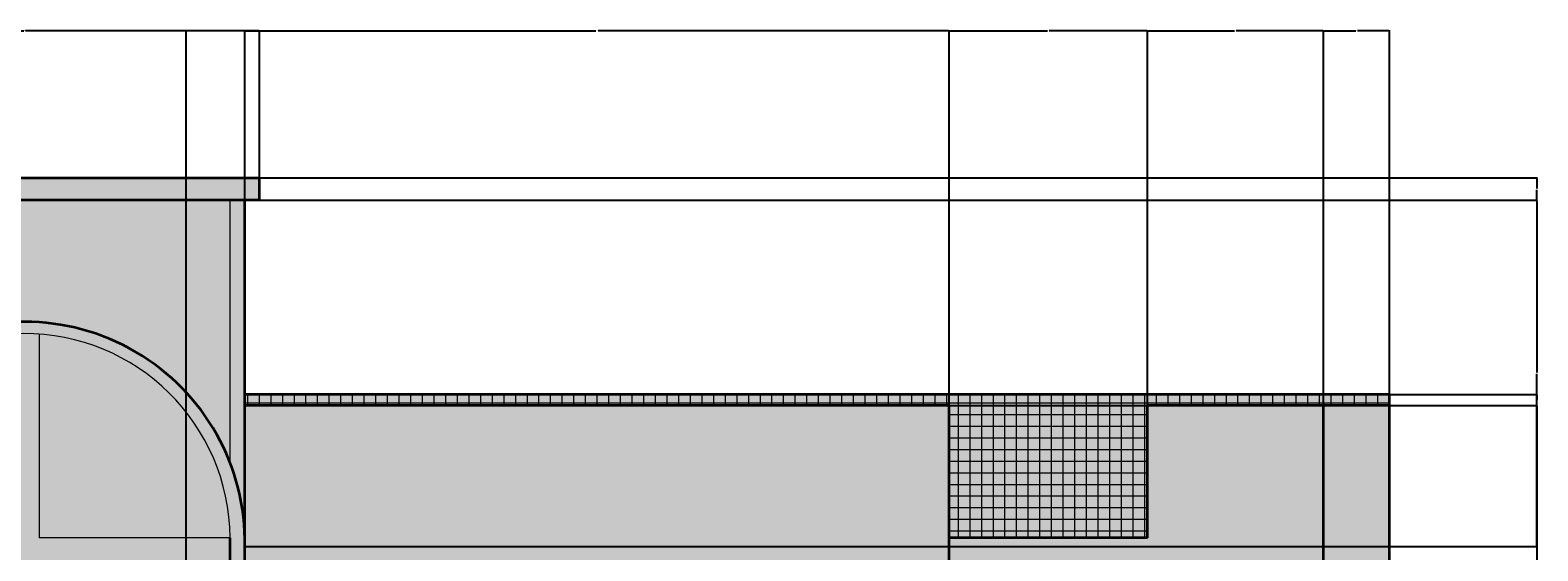
# Model space of a CAD drawing. Units: inches. Extents: x 2794 to 3619, y 522 to 1397.
# Tile 10 of 10: x 3208 to 3619, y 1255 to 1397. Entities that reach past the tile are written whole.
import ezdxf

# ---------------------------------------------------------------- set-up
doc = ezdxf.new("R2010")
doc.units = ezdxf.units.IN
for name, color, linetype, lineweight in [('A-ANNO-DIMS', 2, 'Continuous', 18), ('A-ELEV', 7, 'Continuous', 35), ('A-ELEV-PATT', 8, 'Continuous', 13), ('A-GLAZ', 4, 'Continuous', 18)]:
    doc.layers.add(name, color=color, linetype=linetype, lineweight=lineweight)
doc.styles.get("Standard").update_dxf_attribs({"font": 'arial.ttf'})
doc.dimstyles.get("Standard").update_dxf_attribs({"dimtxt": 0.18, "dimasz": 0.18, "dimexe": 0.18, "dimexo": 0.0625, "dimgap": 0.09, "dimtad": 0, "dimtih": 1, "dimtoh": 1, "dimdec": 4, "dimzin": 0, "dimdsep": 46, "dimtxsty": 'Standard', "dimcen": 0.09, "dimadec": 0, "dimazin": 0, "dimtfac": 1, "dimtdec": 4, "dimtofl": 0, "dimtmove": 0, "dimatfit": 3, "dimfxl": 1, "dimtolj": 1, "dimtzin": 0, "dimarcsym": 0})

# ---------------------------------------------------------------- blocks, each defined once
blk = doc.blocks.new('*D12')
at = {"layer": 'A-ANNO-DIMS', "color": 0, "lineweight": -2, "transparency": 16777216}
for p, q in [((3266.27, 1294.7), (3266.27, 1396.92)), ((3266.45, 1396.74), (3361.99, 1396.74)), ((3458.09, 1396.74), (3362.55, 1396.74)), ((3458.27, 1294.7), (3458.27, 1396.92))]:
    blk.add_line(p, q, dxfattribs=at)
at = {"layer": 'A-ANNO-DIMS', "color": 0, "transparency": 16777216}
for points in [[(3266.45, 1396.77), (3266.45, 1396.71), (3266.27, 1396.74)], [(3458.09, 1396.77), (3458.09, 1396.71), (3458.27, 1396.74)]]:
    blk.add_solid(points, dxfattribs=at)
at = {"layer": 'Defpoints', "color": 0, "transparency": 16777216}
for p in [(3458.27, 1396.74), (3266.27, 1294.64), (3458.27, 1294.64)]:
    blk.add_point(p, dxfattribs=at)
at = {"layer": 'A-ANNO-DIMS', "color": 0, "transparency": 16777216, "insert": (3362.27, 1396.74), "char_height": 0.18, "attachment_point": 5}
blk.add_mtext('\\A1;192', dxfattribs=at)
blk = doc.blocks.new('*D13')
at = {"layer": 'A-ANNO-DIMS', "color": 0, "lineweight": -2, "transparency": 16777216}
for p, q in [((3458.27, 1294.7), (3458.27, 1396.92)), ((3458.45, 1396.74), (3485.05, 1396.74)), ((3512.09, 1396.74), (3485.48, 1396.74)), ((3512.27, 1294.7), (3512.27, 1396.92))]:
    blk.add_line(p, q, dxfattribs=at)
at = {"layer": 'A-ANNO-DIMS', "color": 0, "transparency": 16777216}
for points in [[(3458.45, 1396.77), (3458.45, 1396.71), (3458.27, 1396.74)], [(3512.09, 1396.77), (3512.09, 1396.71), (3512.27, 1396.74)]]:
    blk.add_solid(points, dxfattribs=at)
at = {"layer": 'Defpoints', "color": 0, "transparency": 16777216}
for p in [(3512.27, 1396.74), (3458.27, 1294.64), (3512.27, 1294.64)]:
    blk.add_point(p, dxfattribs=at)
at = {"layer": 'A-ANNO-DIMS', "color": 0, "transparency": 16777216, "insert": (3485.27, 1396.74), "char_height": 0.18, "attachment_point": 5}
blk.add_mtext('\\A1;54', dxfattribs=at)
blk = doc.blocks.new('*D14')
at = {"layer": 'A-ANNO-DIMS', "color": 0, "lineweight": -2, "transparency": 16777216}
for p, q in [((3512.27, 1294.7), (3512.27, 1396.92)), ((3512.45, 1396.74), (3536.04, 1396.74)), ((3560.09, 1396.74), (3536.49, 1396.74)), ((3560.27, 1294.7), (3560.27, 1396.92))]:
    blk.add_line(p, q, dxfattribs=at)
at = {"layer": 'A-ANNO-DIMS', "color": 0, "transparency": 16777216}
for points in [[(3512.45, 1396.77), (3512.45, 1396.71), (3512.27, 1396.74)], [(3560.09, 1396.77), (3560.09, 1396.71), (3560.27, 1396.74)]]:
    blk.add_solid(points, dxfattribs=at)
at = {"layer": 'Defpoints', "color": 0, "transparency": 16777216}
for p in [(3560.27, 1396.74), (3512.27, 1294.64), (3560.27, 1294.64)]:
    blk.add_point(p, dxfattribs=at)
at = {"layer": 'A-ANNO-DIMS', "color": 0, "transparency": 16777216, "insert": (3536.27, 1396.74), "char_height": 0.18, "attachment_point": 5}
blk.add_mtext('\\A1;48', dxfattribs=at)
blk = doc.blocks.new('*D15')
at = {"layer": 'A-ANNO-DIMS', "color": 0, "lineweight": -2, "transparency": 16777216}
for p, q in [((3560.27, 1294.7), (3560.27, 1396.92)), ((3560.45, 1396.74), (3569.06, 1396.74)), ((3578.09, 1396.74), (3569.48, 1396.74)), ((3578.27, 1294.7), (3578.27, 1396.92))]:
    blk.add_line(p, q, dxfattribs=at)
at = {"layer": 'A-ANNO-DIMS', "color": 0, "transparency": 16777216}
for points in [[(3560.45, 1396.77), (3560.45, 1396.71), (3560.27, 1396.74)], [(3578.09, 1396.77), (3578.09, 1396.71), (3578.27, 1396.74)]]:
    blk.add_solid(points, dxfattribs=at)
at = {"layer": 'Defpoints', "color": 0, "transparency": 16777216}
for p in [(3578.27, 1396.74), (3560.27, 1294.64), (3578.27, 1294.64)]:
    blk.add_point(p, dxfattribs=at)
at = {"layer": 'A-ANNO-DIMS', "color": 0, "transparency": 16777216, "insert": (3569.27, 1396.74), "char_height": 0.18, "attachment_point": 5}
blk.add_mtext('\\A1;18', dxfattribs=at)
blk = doc.blocks.new('*D23')
at = {"layer": 'A-ANNO-DIMS', "color": 0, "lineweight": -2, "transparency": 16777216}
for p, q in [((3458.33, 1294.64), (3618.55, 1294.64)), ((3618.37, 1294.46), (3618.37, 1232.82)), ((3618.37, 1170.82), (3618.37, 1232.45)), ((3458.33, 1170.64), (3618.55, 1170.64))]:
    blk.add_line(p, q, dxfattribs=at)
at = {"layer": 'A-ANNO-DIMS', "color": 0, "transparency": 16777216}
for points in [[(3618.34, 1294.46), (3618.4, 1294.46), (3618.37, 1294.64)], [(3618.34, 1170.82), (3618.4, 1170.82), (3618.37, 1170.64)]]:
    blk.add_solid(points, dxfattribs=at)
at = {"layer": 'Defpoints', "color": 0, "transparency": 16777216}
for p in [(3458.27, 1294.64), (3618.37, 1294.64), (3458.27, 1170.64)]:
    blk.add_point(p, dxfattribs=at)
at = {"layer": 'A-ANNO-DIMS', "color": 0, "transparency": 16777216, "insert": (3618.37, 1232.64), "char_height": 0.18, "attachment_point": 5}
blk.add_mtext('\\A1;124', dxfattribs=at)
blk = doc.blocks.new('*D24')
at = {"layer": 'A-ANNO-DIMS', "color": 0, "lineweight": -2, "transparency": 16777216}
for p, q in [((3578.33, 1297.64), (3618.55, 1297.64)), ((3578.33, 1294.64), (3618.55, 1294.64)), ((3618.37, 1297.46), (3618.37, 1296.32)), ((3618.37, 1294.82), (3618.37, 1295.95))]:
    blk.add_line(p, q, dxfattribs=at)
at = {"layer": 'A-ANNO-DIMS', "color": 0, "transparency": 16777216}
for points in [[(3618.34, 1297.46), (3618.4, 1297.46), (3618.37, 1297.64)], [(3618.34, 1294.82), (3618.4, 1294.82), (3618.37, 1294.64)]]:
    blk.add_solid(points, dxfattribs=at)
at = {"layer": 'Defpoints', "color": 0, "transparency": 16777216}
for p in [(3578.27, 1297.64), (3578.27, 1294.64), (3618.37, 1297.64)]:
    blk.add_point(p, dxfattribs=at)
at = {"layer": 'A-ANNO-DIMS', "color": 0, "transparency": 16777216, "insert": (3618.37, 1296.14), "char_height": 0.18, "attachment_point": 5}
blk.add_mtext('\\A1;3', dxfattribs=at)
blk = doc.blocks.new('*D44')
at = {"layer": 'A-ANNO-DIMS', "color": 0, "lineweight": -2, "transparency": 16777216}
for p, q in [((3142.27, 1356.7), (3142.27, 1396.92)), ((3142.45, 1396.74), (3205.99, 1396.74)), ((3270.09, 1396.74), (3206.55, 1396.74)), ((3270.27, 1356.7), (3270.27, 1396.92))]:
    blk.add_line(p, q, dxfattribs=at)
at = {"layer": 'A-ANNO-DIMS', "color": 0, "transparency": 16777216}
for points in [[(3142.45, 1396.77), (3142.45, 1396.71), (3142.27, 1396.74)], [(3270.09, 1396.77), (3270.09, 1396.71), (3270.27, 1396.74)]]:
    blk.add_solid(points, dxfattribs=at)
at = {"layer": 'Defpoints', "color": 0, "transparency": 16777216}
for p in [(3270.27, 1396.74), (3142.27, 1356.64), (3270.27, 1356.64)]:
    blk.add_point(p, dxfattribs=at)
at = {"layer": 'A-ANNO-DIMS', "color": 0, "transparency": 16777216, "insert": (3206.27, 1396.74), "char_height": 0.18, "attachment_point": 5}
blk.add_mtext('\\A1;128', dxfattribs=at)
blk = doc.blocks.new('*D45')
at = {"layer": 'A-ANNO-DIMS', "color": 0, "lineweight": -2, "transparency": 16777216}
for p, q in [((3146.27, 1350.7), (3146.27, 1396.92)), ((3146.45, 1396.74), (3205.99, 1396.74)), ((3266.09, 1396.74), (3206.55, 1396.74)), ((3266.27, 1350.7), (3266.27, 1396.92))]:
    blk.add_line(p, q, dxfattribs=at)
at = {"layer": 'A-ANNO-DIMS', "color": 0, "transparency": 16777216}
for points in [[(3146.45, 1396.77), (3146.45, 1396.71), (3146.27, 1396.74)], [(3266.09, 1396.77), (3266.09, 1396.71), (3266.27, 1396.74)]]:
    blk.add_solid(points, dxfattribs=at)
at = {"layer": 'Defpoints', "color": 0, "transparency": 16777216}
for p in [(3266.27, 1396.74), (3146.27, 1350.64), (3266.27, 1350.64)]:
    blk.add_point(p, dxfattribs=at)
at = {"layer": 'A-ANNO-DIMS', "color": 0, "transparency": 16777216, "insert": (3206.27, 1396.74), "char_height": 0.18, "attachment_point": 5}
blk.add_mtext('\\A1;120', dxfattribs=at)
blk = doc.blocks.new('*D46')
at = {"layer": 'A-ANNO-DIMS', "color": 0, "lineweight": -2, "transparency": 16777216}
for p, q in [((3270.33, 1356.64), (3618.55, 1356.64)), ((3618.37, 1356.46), (3618.37, 1353.82)), ((3618.37, 1350.82), (3618.37, 1353.45)), ((3270.33, 1350.64), (3618.55, 1350.64))]:
    blk.add_line(p, q, dxfattribs=at)
at = {"layer": 'A-ANNO-DIMS', "color": 0, "transparency": 16777216}
for points in [[(3618.34, 1356.46), (3618.4, 1356.46), (3618.37, 1356.64)], [(3618.34, 1350.82), (3618.4, 1350.82), (3618.37, 1350.64)]]:
    blk.add_solid(points, dxfattribs=at)
at = {"layer": 'Defpoints', "color": 0, "transparency": 16777216}
for p in [(3270.27, 1356.64), (3618.37, 1356.64), (3270.27, 1350.64)]:
    blk.add_point(p, dxfattribs=at)
at = {"layer": 'A-ANNO-DIMS', "color": 0, "transparency": 16777216, "insert": (3618.37, 1353.64), "char_height": 0.18, "attachment_point": 5}
blk.add_mtext('\\A1;6', dxfattribs=at)
blk = doc.blocks.new('*D47')
at = {"layer": 'A-ANNO-DIMS', "color": 0, "lineweight": -2, "transparency": 16777216}
for p, q in [((3266.33, 1350.64), (3618.55, 1350.64)), ((3618.37, 1350.46), (3618.37, 1303.62)), ((3618.37, 1256.43), (3618.37, 1303.26)), ((3266.33, 1256.25), (3618.55, 1256.25))]:
    blk.add_line(p, q, dxfattribs=at)
at = {"layer": 'A-ANNO-DIMS', "color": 0, "transparency": 16777216}
for points in [[(3618.34, 1350.46), (3618.4, 1350.46), (3618.37, 1350.64)], [(3618.34, 1256.43), (3618.4, 1256.43), (3618.37, 1256.25)]]:
    blk.add_solid(points, dxfattribs=at)
at = {"layer": 'Defpoints', "color": 0, "transparency": 16777216}
for p in [(3266.27, 1350.64), (3618.37, 1350.64), (3266.27, 1256.25)]:
    blk.add_point(p, dxfattribs=at)
at = {"layer": 'A-ANNO-DIMS', "color": 0, "transparency": 16777216, "insert": (3618.37, 1303.44), "char_height": 0.18, "attachment_point": 5}
blk.add_mtext('\\A1;94.39', dxfattribs=at)
blk = doc.blocks.new('*D56')
at = {"layer": 'A-ANNO-DIMS', "color": 0, "lineweight": -2, "transparency": 16777216}
for p, q in [((3162.27, 664.7), (3162.27, 1396.92)), ((3162.45, 1396.74), (3206.05, 1396.74)), ((3250.09, 1396.74), (3206.49, 1396.74)), ((3250.27, 664.7), (3250.27, 1396.92))]:
    blk.add_line(p, q, dxfattribs=at)
at = {"layer": 'A-ANNO-DIMS', "color": 0, "transparency": 16777216}
for points in [[(3162.45, 1396.77), (3162.45, 1396.71), (3162.27, 1396.74)], [(3250.09, 1396.77), (3250.09, 1396.71), (3250.27, 1396.74)]]:
    blk.add_solid(points, dxfattribs=at)
at = {"layer": 'Defpoints', "color": 0, "transparency": 16777216}
for p in [(3250.27, 1396.74), (3162.27, 664.64), (3250.27, 664.64)]:
    blk.add_point(p, dxfattribs=at)
at = {"layer": 'A-ANNO-DIMS', "color": 0, "transparency": 16777216, "insert": (3206.27, 1396.74), "char_height": 0.18, "attachment_point": 5}
blk.add_mtext('\\A1;88', dxfattribs=at)

msp = doc.modelspace()

# ---------------------------------------------------------------- hatches: boundary and pattern name
at = {"layer": 'A-ELEV-PATT', "transparency": 33554687}
h = msp.add_hatch(color=256, dxfattribs=at)
h.dxf.hatch_style = 1
h.paths.add_polyline_path([(3270.2659, 1356.6351), (3142.2659, 1356.6351), (3142.2659, 1350.6351), (3266.2659, 1350.6351), (3270.2659, 1350.6351)])
h.paths.add_polyline_path([(3266.2659, 1350.6351), (3262.2659, 1350.6351), (3262.2659, 1279.0155, -0.0871789), (3266.2659, 1258.6351)])
h.paths.add_polyline_path([(3150.2659, 1350.6351), (3146.2659, 1350.6351), (3146.2659, 1258.6351, -0.0871789), (3150.2659, 1279.0155)])
h = msp.add_hatch(color=256, dxfattribs=at)
h.dxf.hatch_style = 1
h.paths.add_polyline_path([(3262.2659, 1350.6351), (3150.2659, 1350.6351), (3150.2659, 1279.0155, -0.68639605), (3262.2659, 1279.0155)])
h.paths.add_polyline_path([(3210.2659, 1314.1121), (3210.2659, 1258.6351), (3262.2659, 1258.6351, 0.39146256)])
h.paths.add_polyline_path([(3206.2659, 1314.2551, 0.41222069), (3150.2659, 1258.6351), (3206.2659, 1258.6351)])
h.paths.add_polyline_path([(3262.2659, 1254.6351), (3210.2659, 1254.6351), (3210.2659, 1216.6351), (3262.2659, 1216.6351)])
h.paths.add_polyline_path([(3206.2659, 1254.6351), (3150.2659, 1254.6351), (3150.2659, 1216.6351), (3206.2659, 1216.6351)])
h.paths.add_polyline_path([(3262.2659, 1212.6351), (3210.2659, 1212.6351), (3210.2659, 1186.6351), (3262.2659, 1186.6351)])
h.paths.add_polyline_path([(3206.2659, 1212.6351), (3150.2659, 1212.6351), (3150.2659, 1186.6351), (3206.2659, 1186.6351)])
h.paths.add_polyline_path([(3206.2659, 1182.6351), (3150.2659, 1182.6351), (3150.2659, 1156.6351), (3206.2659, 1156.6351)])
h.paths.add_polyline_path([(3262.2659, 1182.6351), (3210.2659, 1182.6351), (3210.2659, 1156.6351), (3262.2659, 1156.6351)])
h.paths.add_polyline_path([(3262.2659, 1152.6351), (3210.2659, 1152.6351), (3210.2659, 1126.6351), (3262.2659, 1126.6351)])
h.paths.add_polyline_path([(3206.2659, 1152.6351), (3150.2659, 1152.6351), (3150.2659, 1126.6351), (3206.2659, 1126.6351)])
h.paths.add_polyline_path([(3262.2659, 1122.6351), (3210.2659, 1122.6351), (3210.2659, 1096.6351), (3262.2659, 1096.6351)])
h.paths.add_polyline_path([(3206.2659, 1122.6351), (3150.2659, 1122.6351), (3150.2659, 1096.6351), (3206.2659, 1096.6351)])
h.paths.add_polyline_path([(3206.2659, 1092.6351), (3150.2659, 1092.6351), (3150.2659, 1066.6351), (3206.2659, 1066.6351)])
h.paths.add_polyline_path([(3262.2659, 1092.6351), (3210.2659, 1092.6351), (3210.2659, 1066.6351), (3262.2659, 1066.6351)])
h.paths.add_polyline_path([(3262.2659, 1062.6351), (3210.2659, 1062.6351), (3210.2659, 1036.6351), (3262.2659, 1036.6351)])
h.paths.add_polyline_path([(3206.2659, 1062.6351), (3150.2659, 1062.6351), (3150.2659, 1036.6351), (3206.2659, 1036.6351)])
h.paths.add_polyline_path([(3206.2659, 1032.6351), (3150.2659, 1032.6351), (3150.2659, 1006.6351), (3206.2659, 1006.6351)])
h.paths.add_polyline_path([(3262.2659, 1032.6351), (3210.2659, 1032.6351), (3210.2659, 1006.6351), (3262.2659, 1006.6351)])
h.paths.add_polyline_path([(3262.2659, 1002.6351), (3210.2659, 1002.6351), (3210.2659, 976.6351), (3262.2659, 976.6351)])
h.paths.add_polyline_path([(3206.2659, 1002.6351), (3150.2659, 1002.6351), (3150.2659, 976.6351), (3206.2659, 976.6351)])
h.paths.add_polyline_path([(3206.2659, 972.6351), (3150.2659, 972.6351), (3150.2659, 946.6351), (3206.2659, 946.6351)])
h.paths.add_polyline_path([(3206.2659, 942.6351), (3150.2659, 942.6351), (3150.2659, 916.6351), (3206.2659, 916.6351)])
h.paths.add_polyline_path([(3262.2659, 942.6351), (3210.2659, 942.6351), (3210.2659, 916.6351), (3262.2659, 916.6351)])
h.paths.add_polyline_path([(3262.2659, 972.6351), (3210.2659, 972.6351), (3210.2659, 946.6351), (3262.2659, 946.6351)])
h.paths.add_polyline_path([(3262.2659, 912.6351), (3210.2659, 912.6351), (3210.2659, 886.6351), (3262.2659, 886.6351)])
h.paths.add_polyline_path([(3206.2659, 912.6351), (3150.2659, 912.6351), (3150.2659, 886.6351), (3206.2659, 886.6351)])
h.paths.add_polyline_path([(3206.2659, 882.6351), (3150.2659, 882.6351), (3150.2659, 856.6351), (3206.2659, 856.6351)])
h.paths.add_polyline_path([(3262.2659, 882.6351), (3210.2659, 882.6351), (3210.2659, 856.6351), (3262.2659, 856.6351)])
h.paths.add_polyline_path([(3262.2659, 852.6351), (3210.2659, 852.6351), (3210.2659, 826.6351), (3262.2659, 826.6351)])
h.paths.add_polyline_path([(3206.2659, 852.6351), (3150.2659, 852.6351), (3150.2659, 826.6351), (3206.2659, 826.6351)])
h.paths.add_polyline_path([(3206.2659, 822.6351), (3150.2659, 822.6351), (3150.2659, 796.6351), (3206.2659, 796.6351)])
h.paths.add_polyline_path([(3262.2659, 822.6351), (3210.2659, 822.6351), (3210.2659, 796.6351), (3262.2659, 796.6351)])
h.paths.add_polyline_path([(3262.2659, 792.6351), (3210.2659, 792.6351), (3210.2659, 766.6351), (3262.2659, 766.6351)])
h.paths.add_polyline_path([(3206.2659, 792.6351), (3150.2659, 792.6351), (3150.2659, 766.6351), (3206.2659, 766.6351)])
h.paths.add_polyline_path([(3206.2659, 762.6351), (3150.2659, 762.6351), (3150.2659, 736.6351), (3206.2659, 736.6351)])
h.paths.add_polyline_path([(3206.2659, 732.6351), (3150.2659, 732.6351), (3150.2659, 706.6351), (3206.2659, 706.6351)])
h.paths.add_polyline_path([(3262.2659, 732.6351), (3210.2659, 732.6351), (3210.2659, 706.6351), (3262.2659, 706.6351)])
h.paths.add_polyline_path([(3262.2659, 762.6351), (3210.2659, 762.6351), (3210.2659, 736.6351), (3262.2659, 736.6351)])
h = msp.add_hatch(color=256, dxfattribs=at)
h.dxf.hatch_style = 1
h.paths.add_polyline_path([(3146.2659, 1258.6351), (3150.2659, 1258.6351, -0.9932142), (3262.2659, 1258.6351), (3262.2659, 1279.0155, 0.82281137)])
h = msp.add_hatch(color=256, dxfattribs=at)
h.dxf.hatch_style = 1
h.paths.add_polyline_path([(3266.2659, 1258.6351, 0.98030963), (3146.2659, 1258.6351), (3150.2659, 1258.6351, -0.9932142), (3262.2659, 1258.6351), (3262.2659, 1228.6351), (3266.2659, 1228.6351)])
h = msp.add_hatch(color=256, dxfattribs=at)
h.dxf.hatch_style = 1
h.paths.add_polyline_path([(3150.2659, 1257.8725, -0.00340445), (3150.2659, 1258.6351), (3146.2659, 1258.6351), (3146.2659, 1228.6351), (3150.2659, 1228.6351)])
h.paths.add_polyline_path([(3262.2659, 1258.6351), (3210.2659, 1258.6351), (3210.2659, 1314.1121, 0.01787385), (3206.2659, 1314.2551), (3206.2659, 1258.6351), (3150.2659, 1258.6351), (3150.2659, 1254.6351), (3206.2659, 1254.6351), (3206.2659, 1216.6351), (3150.2659, 1216.6351), (3150.2659, 1212.6351), (3206.2659, 1212.6351), (3206.2659, 1186.6351), (3150.2659, 1186.6351), (3150.2659, 1182.6351), (3206.2659, 1182.6351), (3206.2659, 1156.6351), (3150.2659, 1156.6351), (3150.2659, 1152.6351), (3206.2659, 1152.6351), (3206.2659, 1126.6351), (3150.2659, 1126.6351), (3150.2659, 1122.6351), (3206.2659, 1122.6351), (3206.2659, 1096.6351), (3150.2659, 1096.6351), (3150.2659, 1092.6351), (3206.2659, 1092.6351), (3206.2659, 1066.6351), (3150.2659, 1066.6351), (3150.2659, 1062.6351), (3206.2659, 1062.6351), (3206.2659, 1036.6351), (3150.2659, 1036.6351), (3150.2659, 1032.6351), (3206.2659, 1032.6351), (3206.2659, 1006.6351), (3150.2659, 1006.6351), (3150.2659, 1002.6351), (3206.2659, 1002.6351), (3206.2659, 976.6351), (3150.2659, 976.6351), (3150.2659, 972.6351), (3206.2659, 972.6351), (3206.2659, 946.6351), (3150.2659, 946.6351), (3150.2659, 942.6351), (3206.2659, 942.6351), (3206.2659, 916.6351), (3150.2659, 916.6351), (3150.2659, 912.6351), (3206.2659, 912.6351), (3206.2659, 886.6351), (3150.2659, 886.6351), (3150.2659, 882.6351), (3206.2659, 882.6351), (3206.2659, 856.6351), (3150.2659, 856.6351), (3150.2659, 852.6351), (3206.2659, 852.6351), (3206.2659, 826.6351), (3150.2659, 826.6351), (3150.2659, 822.6351), (3206.2659, 822.6351), (3206.2659, 796.6351), (3150.2659, 796.6351), (3150.2659, 792.6351), (3206.2659, 792.6351), (3206.2659, 766.6351), (3150.2659, 766.6351), (3150.2659, 762.6351), (3206.2659, 762.6351), (3206.2659, 736.6351), (3150.2659, 736.6351), (3150.2659, 732.6351), (3206.2659, 732.6351), (3206.2659, 706.6351), (3150.2659, 706.6351), (3150.2659, 702.6351), (3262.2659, 702.6351), (3262.2659, 706.6351), (3210.2659, 706.6351), (3210.2659, 732.6351), (3262.2659, 732.6351), (3262.2659, 736.6351), (3210.2659, 736.6351), (3210.2659, 762.6351), (3262.2659, 762.6351), (3262.2659, 766.6351), (3210.2659, 766.6351), (3210.2659, 792.6351), (3262.2659, 792.6351), (3262.2659, 796.6351), (3210.2659, 796.6351), (3210.2659, 822.6351), (3262.2659, 822.6351), (3262.2659, 826.6351), (3210.2659, 826.6351), (3210.2659, 852.6351), (3262.2659, 852.6351), (3262.2659, 856.6351), (3210.2659, 856.6351), (3210.2659, 882.6351), (3262.2659, 882.6351), (3262.2659, 886.6351), (3210.2659, 886.6351), (3210.2659, 912.6351), (3262.2659, 912.6351), (3262.2659, 916.6351), (3210.2659, 916.6351), (3210.2659, 942.6351), (3262.2659, 942.6351), (3262.2659, 946.6351), (3210.2659, 946.6351), (3210.2659, 972.6351), (3262.2659, 972.6351), (3262.2659, 976.6351), (3210.2659, 976.6351), (3210.2659, 1002.6351), (3262.2659, 1002.6351), (3262.2659, 1006.6351), (3210.2659, 1006.6351), (3210.2659, 1032.6351), (3262.2659, 1032.6351), (3262.2659, 1036.6351), (3210.2659, 1036.6351), (3210.2659, 1062.6351), (3262.2659, 1062.6351), (3262.2659, 1066.6351), (3210.2659, 1066.6351), (3210.2659, 1092.6351), (3262.2659, 1092.6351), (3262.2659, 1096.6351), (3210.2659, 1096.6351), (3210.2659, 1122.6351), (3262.2659, 1122.6351), (3262.2659, 1126.6351), (3210.2659, 1126.6351), (3210.2659, 1152.6351), (3262.2659, 1152.6351), (3262.2659, 1156.6351), (3210.2659, 1156.6351), (3210.2659, 1182.6351), (3262.2659, 1182.6351), (3262.2659, 1186.6351), (3210.2659, 1186.6351), (3210.2659, 1212.6351), (3262.2659, 1212.6351), (3262.2659, 1216.6351), (3210.2659, 1216.6351), (3210.2659, 1254.6351), (3262.2659, 1254.6351)])
at = {"layer": 'A-ELEV-PATT'}
h = msp.add_hatch(dxfattribs=at)
h.set_pattern_fill('NET', color=256)
h.paths.add_polyline_path([(2834.2659, 1297.6351), (2834.2659, 1294.6351), (2900.2659, 1294.6351), (2900.2659, 1258.6351), (2954.2659, 1258.6351), (2954.2659, 1294.6351), (3146.2659, 1294.6351), (3146.2659, 1297.6351)])
h.paths.add_polyline_path([(3512.2659, 1258.6351), (3512.2659, 1294.6351), (3578.2659, 1294.6351), (3578.2659, 1297.6351), (3266.2659, 1297.6351), (3266.2659, 1294.6351), (3458.2659, 1294.6351), (3458.2659, 1258.6351)])
at = {"layer": 'A-ELEV-PATT', "transparency": 33554687}
h = msp.add_hatch(color=256, dxfattribs=at)
h.dxf.hatch_style = 1
h.paths.add_polyline_path([(3578.2659, 1294.6351), (3560.2659, 1294.6351), (3560.2659, 642.6351), (3578.2659, 642.6351)])
h.paths.add_polyline_path([(2852.2659, 1294.6351), (2834.2659, 1294.6351), (2834.2659, 642.6351), (2852.2659, 642.6351)])
h = msp.add_hatch(color=256, dxfattribs=at)
h.dxf.hatch_style = 1
h.paths.add_polyline_path([(2852.2659, 1294.6351), (2834.2659, 1294.6351), (2834.2659, 562.6351), (2852.2659, 562.6351)])
h.paths.add_polyline_path([(3578.2659, 1294.6351), (3560.2659, 1294.6351), (3560.2659, 562.6351), (3578.2659, 562.6351)])
h = msp.add_hatch(color=256, dxfattribs=at)
h.dxf.hatch_style = 1
h.paths.add_polyline_path([(2852.2659, 1246.6351), (2954.2659, 1246.6351), (2954.2659, 1258.6351), (2900.2659, 1258.6351), (2900.2659, 1294.6351), (2852.2659, 1294.6351)])
h.paths.add_polyline_path([(3512.2659, 1294.6351), (3512.2659, 1258.6351), (3458.2659, 1258.6351), (3458.2659, 1246.6351), (3560.2659, 1246.6351), (3560.2659, 1294.6351)])
h.paths.add_polyline_path([(2954.2659, 1114.6351), (2954.2659, 1126.6351), (2852.2659, 1126.6351), (2852.2659, 1114.6351)])
h.paths.add_polyline_path([(3560.2659, 1114.6351), (3560.2659, 1126.6351), (3458.2659, 1126.6351), (3458.2659, 1114.6351)])
h.paths.add_polyline_path([(3560.2659, 982.6351), (3560.2659, 994.6351), (3458.2659, 994.6351), (3458.2659, 982.6351)])
h.paths.add_polyline_path([(2954.2659, 982.6351), (2954.2659, 994.6351), (2852.2659, 994.6351), (2852.2659, 982.6351)])
h.paths.add_polyline_path([(2852.2659, 862.6351), (2852.2659, 850.6351), (2954.2659, 850.6351), (2954.2659, 862.6351)])
h.paths.add_polyline_path([(2852.2659, 730.6351), (2852.2659, 718.6351), (2954.2659, 718.6351), (2954.2659, 730.6351)])
h.paths.add_polyline_path([(3560.2659, 718.6351), (3560.2659, 730.6351), (3458.2659, 730.6351), (3458.2659, 718.6351)])
h.paths.add_polyline_path([(3560.2659, 850.6351), (3560.2659, 862.6351), (3458.2659, 862.6351), (3458.2659, 850.6351)])
h = msp.add_hatch(color=256, dxfattribs=at)
h.dxf.hatch_style = 1
h.paths.add_polyline_path([(3146.2659, 1096.6351), (3146.2659, 1126.6351), (2954.2659, 1126.6351), (2954.2659, 1096.6351)])
h.paths.add_polyline_path([(3458.2659, 1096.6351), (3458.2659, 1126.6351), (3266.2659, 1126.6351), (3266.2659, 1096.6351)])
h.paths.add_polyline_path([(3458.2659, 964.6351), (3458.2659, 994.6351), (3266.2659, 994.6351), (3266.2659, 964.6351)])
h.paths.add_polyline_path([(3146.2659, 964.6351), (3146.2659, 994.6351), (2954.2659, 994.6351), (2954.2659, 964.6351)])
h.paths.add_polyline_path([(3458.2659, 832.6351), (3458.2659, 862.6351), (3266.2659, 862.6351), (3266.2659, 832.6351)])
h.paths.add_polyline_path([(3146.2659, 832.6351), (3146.2659, 862.6351), (2954.2659, 862.6351), (2954.2659, 832.6351)])
h.paths.add_polyline_path([(3458.2659, 700.6351), (3458.2659, 730.6351), (3266.2659, 730.6351), (3266.2659, 700.6351)])
h.paths.add_polyline_path([(3146.2659, 700.6351), (3146.2659, 730.6351), (2954.2659, 730.6351), (2954.2659, 700.6351)])
h.paths.add_polyline_path([(3266.2659, 1294.6351), (3266.2659, 1258.6351), (3266.2659, 1228.6351), (3458.2659, 1228.6351), (3458.2659, 1294.6351)])
h.paths.add_polyline_path([(3146.2659, 1228.6351), (3146.2659, 1256.2485, -0.00994307), (3146.2659, 1258.6351), (3146.2659, 1294.6351), (2954.2659, 1294.6351), (2954.2659, 1228.6351)])
h = msp.add_hatch(color=256, dxfattribs=at)
h.dxf.hatch_style = 1
h.paths.add_polyline_path([(3266.2659, 1297.6351), (3266.2659, 1294.6351), (3458.2659, 1294.6351), (3458.2659, 1258.6351), (3512.2659, 1258.6351), (3512.2659, 1294.6351), (3578.2659, 1294.6351), (3578.2659, 1297.6351)])

# ---------------------------------------------------------------- linework, layer by layer
at = {"layer": 'A-ELEV'}
for p, q in [((3270.2659, 1356.6351), (3142.2659, 1356.6351)), ((3270.2659, 1350.6351), (3270.2659, 1356.6351)), ((3266.2659, 1350.6351), (3142.2659, 1350.6351)), ((3266.2659, 1258.6351), (3266.2659, 1350.6351)), ((3270.2659, 1350.6351), (3266.2659, 1350.6351)), ((3578.2659, 1297.6351), (3266.2659, 1297.6351)), ((3458.2659, 1294.6351), (3266.2659, 1294.6351)), ((3458.2659, 598.6351), (3458.2659, 1294.6351)), ((3578.2659, 1294.6351), (3512.2659, 1294.6351)), ((3512.2659, 1258.6351), (3512.2659, 1294.6351)), ((3560.2659, 562.6351), (3560.2659, 1294.6351)), ((3578.2659, 562.6351), (3578.2659, 1297.6351)), ((3262.2659, 598.6351), (3262.2659, 1258.6351)), ((3266.2659, 598.6351), (3266.2659, 1258.6351)), ((3512.2659, 1258.6351), (3458.2659, 1258.6351))]:
    msp.add_line(p, q, dxfattribs=at)
msp.add_arc((3206.2659, 1257.4418), 60.0119, 358.860645, 181.139355, dxfattribs=at)
at = {"layer": 'A-GLAZ'}
for p, q in [((3262.2659, 1350.6351), (3248.8399, 1350.6351)), ((3262.2659, 1279.0155), (3262.2659, 1350.6351)), ((3208.2659, 1317.4537), (3208.2659, 1317.4203)), ((3210.2659, 1314.2194), (3210.2659, 1258.6351)), ((3262.2659, 1258.6351), (3210.2659, 1258.6351))]:
    msp.add_line(p, q, dxfattribs=at)
msp.add_arc((3206.2659, 1258.2538), 56.0013, 0.39012, 180.39012, dxfattribs=at)

# ---------------------------------------------------------------- dimensions: what is measured, and where the dimension line sits
at = {"layer": 'A-ANNO-DIMS'}
for base, p1, p2, picture, middle in [((3270.2659, 1396.7351), (3142.2659, 1356.6351), (3270.2659, 1356.6351), '*D44', (3206.2659, 1396.7351)), ((3266.2659, 1396.7351), (3146.2659, 1350.6351), (3266.2659, 1350.6351), '*D45', (3206.2659, 1396.7351)), ((3250.2659, 1396.7351), (3162.2659, 664.6351), (3250.2659, 664.6351), '*D56', (3206.2659, 1396.7351)), ((3458.2659, 1396.7351), (3266.2659, 1294.6351), (3458.2659, 1294.6351), '*D12', (3362.2659, 1396.7351)), ((3512.2659, 1396.7351), (3458.2659, 1294.6351), (3512.2659, 1294.6351), '*D13', (3485.2659, 1396.7351)), ((3560.2659, 1396.7351), (3512.2659, 1294.6351), (3560.2659, 1294.6351), '*D14', (3536.2659, 1396.7351)), ((3578.2659, 1396.7351), (3560.2659, 1294.6351), (3578.2659, 1294.6351), '*D15', (3569.2659, 1396.7351))]:
    dim = msp.add_linear_dim(base=base, p1=p1, p2=p2, dimstyle='Standard', override={"dimdec": 0, "dimlfac": 1, "dimrnd": 0, "dimzin": 0, "dimdsep": 46, "dimlunit": 2}, dxfattribs=at)
    dim.commit()
    dim.dimension.update_dxf_attribs({"geometry": picture, "text_midpoint": middle})
for base, p1, p2, override, picture, middle in [((3618.3659, 1356.6351), (3270.2659, 1350.6351), (3270.2659, 1356.6351), {"dimdec": 0, "dimlfac": 1, "dimrnd": 0, "dimzin": 0, "dimdsep": 46, "dimlunit": 2}, '*D46', (3618.3659, 1353.6351)), ((3618.3659, 1350.6351), (3266.2659, 1256.2485), (3266.2659, 1350.6351), {"dimdec": 2, "dimlfac": 1, "dimrnd": 0, "dimzin": 0, "dimdsep": 46, "dimlunit": 2}, '*D47', (3618.3659, 1303.4418)), ((3618.3659, 1294.6351), (3458.2659, 1170.6351), (3458.2659, 1294.6351), {"dimdec": 0, "dimlfac": 1, "dimrnd": 0, "dimzin": 0, "dimdsep": 46, "dimlunit": 2}, '*D23', (3618.3659, 1232.6351)), ((3618.3659, 1297.6351), (3578.2659, 1294.6351), (3578.2659, 1297.6351), {"dimdec": 0, "dimlfac": 1, "dimrnd": 0, "dimzin": 0, "dimdsep": 46, "dimlunit": 2}, '*D24', (3618.3659, 1296.1351))]:
    dim = msp.add_linear_dim(base=base, p1=p1, p2=p2, angle=90, dimstyle='Standard', override=override, dxfattribs=at)
    dim.commit()
    dim.dimension.update_dxf_attribs({"geometry": picture, "text_midpoint": middle})

doc.saveas('drawing.dxf')
